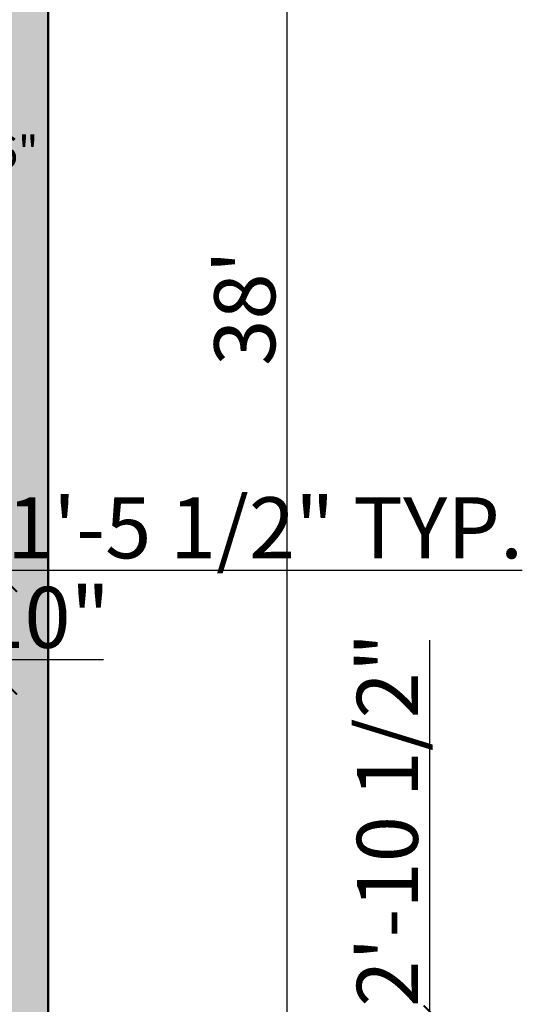
# Model space of a CAD drawing. Units: inches. Extents: x 2419 to 2878, y 1068 to 1713.
# Tile 13 of 20: x 2775 to 2878, y 1207 to 1409. Entities that reach past the tile are written whole.
import ezdxf

# ---------------------------------------------------------------- set-up
doc = ezdxf.new("R2010")
doc.units = ezdxf.units.IN
for name, color, linetype, lineweight in [('A-ANNO-DIMS', 2, 'Continuous', 18), ('A-AREA-IDEN', 7, 'Continuous', 18), ('A-FLOR-PRKG-PATT', 1, 'Continuous', 13), ('A-FURN-PATT', 254, 'Continuous', 13), ('A-WALL', 7, 'Continuous', 50)]:
    doc.layers.add(name, color=color, linetype=linetype, lineweight=lineweight)
doc.layers.add('A-FLOR-FIXT-PATT', color=254, linetype='Continuous', lineweight=13, true_color=0xd7ebd2)
doc.layers.add('A-WALL-PATT', color=18, linetype='Continuous', lineweight=13, true_color=0x000000)
doc.styles.get("Standard").update_dxf_attribs({"font": 'arial.ttf'})
doc.dimstyles.new('ISO-25', dxfattribs={"dimtxt": 12.5, "dimasz": 2.5, "dimexe": 1.25, "dimexo": 0.625, "dimtad": 1, "dimdec": 0, "dimlunit": 4, "dimtxsty": 'Standard', "dimblk": 'ARCHTICK', "dimcen": 2.5, "dimse1": 1, "dimse2": 1, "dimclrd": 4, "dimadec": 0, "dimazin": 0, "dimtfac": 1, "dimtdec": 0, "dimtmove": 0, "dimatfit": 3, "dimfxl": 1, "dimarcsym": 0})

# ---------------------------------------------------------------- blocks, each defined once
blk = doc.blocks.new('_ArchTick')
at = {"color": 0, "linetype": 'ByBlock', "const_width": 0.15}
blk.add_lwpolyline([(-0.5, -0.5), (0.5, 0.5)], dxfattribs=at)
blk = doc.blocks.new('*D17')
at = {"layer": 'A-ANNO-DIMS', "color": 0, "lineweight": -2, "transparency": 16777216}
blk.add_line((2829.44, 1577.81), (2829.44, 1121.81), dxfattribs=at)
at = {"layer": 'Defpoints', "color": 0, "transparency": 16777216}
for p in [(2780.51, 1577.81), (2780.51, 1121.81), (2829.44, 1121.81)]:
    blk.add_point(p, dxfattribs=at)
at = {"layer": 'A-ANNO-DIMS', "color": 0, "lineweight": -2, "transparency": 16777216, "xscale": 2.5, "yscale": 2.5, "zscale": 2.5}
for p, rotation in [((2829.44, 1577.81), 90), ((2829.44, 1121.81), 270)]:
    blk.add_blockref('_ArchTick', p, dxfattribs=dict(at, rotation=rotation))
at = {"layer": 'A-ANNO-DIMS', "color": 0, "transparency": 16777216, "insert": (2822.42, 1349.81), "char_height": 12.5, "attachment_point": 5, "rotation": 90}
blk.add_mtext("38'", dxfattribs=at)
blk = doc.blocks.new('*D18')
at = {"layer": 'A-ANNO-DIMS', "color": 4, "lineweight": -2, "transparency": 16777216}
for p, q in [((2772.91, 1292.99), (2772.91, 1271.99)), ((2772.91, 1271.99), (2772.91, 1133))]:
    blk.add_line(p, q, dxfattribs=at)
at = {"layer": 'Defpoints', "color": 0, "transparency": 16777216}
for p in [(2769.76, 1292.99), (2769.76, 1271.99), (2772.91, 1271.99)]:
    blk.add_point(p, dxfattribs=at)
at = {"layer": 'A-ANNO-DIMS', "color": 4, "lineweight": -2, "transparency": 16777216, "xscale": 2.5, "yscale": 2.5, "zscale": 2.5}
for p, rotation in [((2772.91, 1292.99), 90), ((2772.91, 1271.99), 270)]:
    blk.add_blockref('_ArchTick', p, dxfattribs=dict(at, rotation=rotation))
at = {"layer": 'A-ANNO-DIMS', "color": 0, "transparency": 16777216, "insert": (2765.82, 1201.24), "char_height": 12.5, "attachment_point": 5, "rotation": 90}
blk.add_mtext('CHAIR 1\'-9" TYP.', dxfattribs=at)
blk = doc.blocks.new('*D19')
at = {"layer": 'A-ANNO-DIMS', "color": 4, "lineweight": -2, "transparency": 16777216}
for p, q in [((2752.42, 1296.14), (2769.76, 1296.14)), ((2769.76, 1296.14), (2877.65, 1296.14))]:
    blk.add_line(p, q, dxfattribs=at)
at = {"layer": 'Defpoints', "color": 0, "transparency": 16777216}
for p in [(2769.76, 1296.14), (2752.42, 1292.99), (2769.76, 1292.99)]:
    blk.add_point(p, dxfattribs=at)
at = {"layer": 'A-ANNO-DIMS', "color": 4, "lineweight": -2, "transparency": 16777216, "xscale": 2.5, "yscale": 2.5, "zscale": 2.5, "rotation": 180}
blk.add_blockref('_ArchTick', (2752.42, 1296.14), dxfattribs=at)
at = {"layer": 'A-ANNO-DIMS', "color": 4, "lineweight": -2, "transparency": 16777216, "xscale": 2.5, "yscale": 2.5, "zscale": 2.5}
blk.add_blockref('_ArchTick', (2769.76, 1296.14), dxfattribs=at)
at = {"layer": 'A-ANNO-DIMS', "color": 0, "transparency": 16777216, "insert": (2824.95, 1303.22), "char_height": 12.5, "attachment_point": 5}
blk.add_mtext('1\'-5 1/2" TYP.', dxfattribs=at)
blk = doc.blocks.new('*D33')
at = {"layer": 'A-ANNO-DIMS', "color": 4, "lineweight": -2, "transparency": 16777216}
for p, q in [((2710.85, 1277.89), (2744.94, 1277.89)), ((2744.94, 1277.89), (2791.85, 1277.89))]:
    blk.add_line(p, q, dxfattribs=at)
at = {"layer": 'Defpoints', "color": 0, "transparency": 16777216}
for p in [(2744.94, 1277.89), (2710.85, 1272.77), (2744.94, 1272.77)]:
    blk.add_point(p, dxfattribs=at)
at = {"layer": 'A-ANNO-DIMS', "color": 4, "lineweight": -2, "transparency": 16777216, "xscale": 2.5, "yscale": 2.5, "zscale": 2.5, "rotation": 180}
blk.add_blockref('_ArchTick', (2710.85, 1277.89), dxfattribs=at)
at = {"layer": 'A-ANNO-DIMS', "color": 4, "lineweight": -2, "transparency": 16777216, "xscale": 2.5, "yscale": 2.5, "zscale": 2.5}
blk.add_blockref('_ArchTick', (2744.94, 1277.89), dxfattribs=at)
at = {"layer": 'A-ANNO-DIMS', "color": 0, "transparency": 16777216, "insert": (2769.65, 1284.89), "char_height": 12.5, "attachment_point": 5}
blk.add_mtext('2\'-10"', dxfattribs=at)
blk = doc.blocks.new('*D37')
at = {"layer": 'A-ANNO-DIMS', "color": 4, "lineweight": -2, "transparency": 16777216}
for p, q in [((2736.32, 1605.01), (2771.51, 1605.01)), ((2771.51, 1605.01), (2818.42, 1605.01))]:
    blk.add_line(p, q, dxfattribs=at)
at = {"layer": 'Defpoints', "color": 0, "transparency": 16777216}
for p in [(2771.51, 1605.01), (2736.32, 1205.81), (2771.51, 1205.81)]:
    blk.add_point(p, dxfattribs=at)
at = {"layer": 'A-ANNO-DIMS', "color": 4, "lineweight": -2, "transparency": 16777216, "xscale": 2.5, "yscale": 2.5, "zscale": 2.5, "rotation": 180}
blk.add_blockref('_ArchTick', (2736.32, 1605.01), dxfattribs=at)
at = {"layer": 'A-ANNO-DIMS', "color": 4, "lineweight": -2, "transparency": 16777216, "xscale": 2.5, "yscale": 2.5, "zscale": 2.5}
blk.add_blockref('_ArchTick', (2771.51, 1605.01), dxfattribs=at)
at = {"layer": 'A-ANNO-DIMS', "color": 0, "transparency": 16777216, "insert": (2796.22, 1611.91), "char_height": 12.5, "attachment_point": 5}
blk.add_mtext('2\'-11"', dxfattribs=at)
blk = doc.blocks.new('*D40')
at = {"layer": 'A-ANNO-DIMS', "color": 4, "lineweight": -2, "transparency": 16777216}
for p, q in [((2858.71, 1205.81), (2858.71, 1281.84)), ((2858.71, 1171.28), (2858.71, 1205.81))]:
    blk.add_line(p, q, dxfattribs=at)
at = {"layer": 'Defpoints', "color": 0, "transparency": 16777216}
for p in [(2736.32, 1205.81), (2858.71, 1205.81), (2736.32, 1171.28)]:
    blk.add_point(p, dxfattribs=at)
at = {"layer": 'A-ANNO-DIMS', "color": 4, "lineweight": -2, "transparency": 16777216, "xscale": 2.5, "yscale": 2.5, "zscale": 2.5}
for p, rotation in [((2858.71, 1205.81), 90), ((2858.71, 1171.28), 270)]:
    blk.add_blockref('_ArchTick', p, dxfattribs=dict(at, rotation=rotation))
at = {"layer": 'A-ANNO-DIMS', "color": 0, "transparency": 16777216, "insert": (2851.63, 1245.08), "char_height": 12.5, "attachment_point": 5, "rotation": 90}
blk.add_mtext('2\'-10 1/2"', dxfattribs=at)
blk = doc.blocks.new('*D51')
at = {"layer": 'A-ANNO-DIMS', "color": 4, "lineweight": -2, "transparency": 16777216}
for p, q in [((2738.51, 1079.92), (2771.51, 1079.92)), ((2771.51, 1079.92), (2808.71, 1079.92))]:
    blk.add_line(p, q, dxfattribs=at)
at = {"layer": 'Defpoints', "color": 0, "transparency": 16777216}
for p in [(2738.51, 1447.89), (2771.51, 1437.39), (2771.51, 1079.92)]:
    blk.add_point(p, dxfattribs=at)
at = {"layer": 'A-ANNO-DIMS', "color": 4, "lineweight": -2, "transparency": 16777216, "xscale": 2.5, "yscale": 2.5, "zscale": 2.5, "rotation": 180}
blk.add_blockref('_ArchTick', (2738.51, 1079.92), dxfattribs=at)
at = {"layer": 'A-ANNO-DIMS', "color": 4, "lineweight": -2, "transparency": 16777216, "xscale": 2.5, "yscale": 2.5, "zscale": 2.5}
blk.add_blockref('_ArchTick', (2771.51, 1079.92), dxfattribs=at)
at = {"layer": 'A-ANNO-DIMS', "color": 0, "transparency": 16777216, "insert": (2791.36, 1086.93), "char_height": 12.5, "attachment_point": 5}
blk.add_mtext('2\'-9"', dxfattribs=at)

msp = doc.modelspace()

# ---------------------------------------------------------------- hatches: boundary and pattern name
at = {"layer": 'A-FLOR-FIXT-PATT'}
h = msp.add_hatch(color=256, dxfattribs=at)
h.dxf.hatch_style = 1
h.paths.add_polyline_path([(2771.51, 1458.39), (2763.51, 1458.39), (2763.51, 1437.39), (2771.51, 1437.39)])
h.paths.add_polyline_path([(2770.51, 1456.39, 0.5), (2769.51, 1457.39), (2765.51, 1457.39, 0.5), (2764.51, 1456.39), (2764.51, 1439.39, 0.5), (2765.51, 1438.39), (2769.51, 1438.39, 0.5), (2770.51, 1439.39)], flags=16)
h.paths.add_polyline_path([(2706.38, 1408.81), (2685.38, 1408.81), (2685.38, 1400.81), (2706.38, 1400.81)])
h.paths.add_polyline_path([(2704.38, 1401.81, 0.5), (2705.38, 1402.81), (2705.38, 1406.81, 0.5), (2704.38, 1407.81), (2687.38, 1407.81, 0.5), (2686.38, 1406.81), (2686.38, 1402.81, 0.5), (2687.38, 1401.81)], flags=16)
h.paths.add_polyline_path([(2574.48, 1207.45), (2633.94, 1207.45), (2633.94, 1217.37), (2574.48, 1217.37)], flags=9)
h.paths.add_polyline_path([(2574.45, 1217.83), (2610.47, 1217.83), (2610.47, 1227.88), (2574.45, 1227.88)], flags=9)
h.paths.add_polyline_path([(2672.43, 1304.02), (2718.62, 1304.02), (2718.62, 1313.94), (2672.43, 1313.94)], flags=9)
h.paths.add_polyline_path([(2672.4, 1314.4), (2750.13, 1314.4), (2750.13, 1324.45), (2672.4, 1324.45)], flags=9)
h.paths.add_polyline_path([(2500.43, 1374.44), (2544.8, 1374.44), (2544.8, 1384.36), (2500.43, 1384.36)], flags=9)
h.paths.add_polyline_path([(2500.41, 1384.82), (2566.08, 1384.82), (2566.08, 1394.87), (2500.41, 1394.87)], flags=9)
h.paths.add_polyline_path([(2738.93, 1376.75), (2778.27, 1376.75), (2778.27, 1386.67), (2738.93, 1386.67)], flags=9)
h.paths.add_polyline_path([(2659.12, 1357.8), (2703.49, 1357.8), (2703.49, 1367.72), (2659.12, 1367.72)], flags=9)
h.paths.add_polyline_path([(2659.1, 1368.18), (2694.11, 1368.18), (2694.11, 1378.23), (2659.1, 1378.23)], flags=9)
h.paths.add_polyline_path([(2730.12, 1466.07), (2769.46, 1466.07), (2769.46, 1475.99), (2730.12, 1475.99)], flags=9)
h.paths.add_polyline_path([(2730.1, 1476.45), (2765.12, 1476.45), (2765.12, 1486.5), (2730.1, 1486.5)], flags=9)
h.paths.add_polyline_path([(2730.38, 1518.65), (2761.48, 1518.65), (2761.48, 1528.57), (2730.38, 1528.57)], flags=9)
h.paths.add_polyline_path([(2730.36, 1529.03), (2780.96, 1529.03), (2780.96, 1539.07), (2730.36, 1539.07)], flags=9)
h.paths.add_polyline_path([(2629.32, 1455.19), (2688.78, 1455.19), (2688.78, 1465.11), (2629.32, 1465.11)], flags=9)
h.paths.add_polyline_path([(2629.3, 1465.57), (2681.9, 1465.57), (2681.9, 1475.62), (2629.3, 1475.62)], flags=9)
h.paths.add_polyline_path([(2513.23, 1456.48), (2562.63, 1456.48), (2562.63, 1466.4), (2513.23, 1466.4)], flags=9)
h.paths.add_polyline_path([(2513.21, 1466.86), (2556.26, 1466.86), (2556.26, 1476.91), (2513.21, 1476.91)], flags=9)
h.paths.add_polyline_path([(2488.87, 1521.54), (2519.97, 1521.54), (2519.97, 1531.46), (2488.87, 1531.46)], flags=9)
h.paths.add_polyline_path([(2536.55, 1543.51), (2580.92, 1543.51), (2580.92, 1553.43), (2536.55, 1553.43)], flags=9)
h.paths.add_polyline_path([(2536.56, 1553.92), (2573.53, 1553.92), (2573.53, 1563.8), (2536.56, 1563.8)], flags=9)
at = {"layer": 'A-FLOR-PRKG-PATT'}
h = msp.add_hatch(color=256, dxfattribs=at)
h.dxf.hatch_style = 1
edge = h.paths.add_edge_path()
edge.add_ellipse((2561.37, 1279.45), major_axis=(3.99, 0), ratio=0.842304, start_angle=0.6466, end_angle=90)
edge.add_line((2561.37, 1282.81), (2511.57, 1282.81))
edge.add_ellipse((2511.57, 1279.45), major_axis=(3.99, 0), ratio=0.842304, start_angle=90, end_angle=179.3534)
edge.add_ellipse((10560.89, 1188.62), major_axis=(-8054.03, 0), ratio=0.8423039, start_angle=-0.646554, end_angle=-0.628237)
edge.add_ellipse((2509.23, 1276.91), major_axis=(1.69, 0), ratio=0.842304, start_angle=179.3718, end_angle=248.4648)
edge.add_ellipse((10560.33, 1188.62), major_axis=(8052.29, 0), ratio=0.8423039, start_angle=179.353446, end_angle=179.381357, ccw=False)
edge.add_ellipse((2511.01, 1279.45), major_axis=(2.25, 0), ratio=0.842304, start_angle=90, end_angle=179.3534, ccw=False)
edge.add_line((2511.01, 1281.35), (2561.94, 1281.35))
edge.add_ellipse((2561.94, 1279.45), major_axis=(-2.25, 0), ratio=0.842304, start_angle=180.6466, end_angle=270, ccw=False)
edge.add_ellipse((-5487.38, 1188.62), major_axis=(8052.29, 0), ratio=0.8423039, start_angle=0.528271, end_angle=0.646554, ccw=False)
edge.add_ellipse((2563.71, 1276.91), major_axis=(-1.69, 0), ratio=0.842304, start_angle=111.5352, end_angle=180.6282)
edge.add_ellipse((-5487.95, 1188.62), major_axis=(-8054.03, 0), ratio=0.8423039, start_angle=180.628237, end_angle=180.646554)
edge = h.paths.add_edge_path()
edge.add_ellipse((2564.91, 1261.91), major_axis=(-1.12, 0), ratio=0.842304, start_angle=180, end_angle=270)
edge.add_line((2564.91, 1262.86), (2564.43, 1262.86))
edge.add_ellipse((-5487.38, 1188.62), major_axis=(8052.29, 0), ratio=0.8423039, start_angle=0.383867, end_angle=0.528271, ccw=False)
edge.add_line((2564.65, 1242.56), (2564.91, 1242.56))
edge.add_ellipse((2564.91, 1243.51), major_axis=(-1.12, 0), ratio=0.842304, start_angle=90, end_angle=180)
edge.add_line((2566.03, 1243.51), (2566.03, 1261.91))
edge = h.paths.add_edge_path()
edge.add_ellipse((2564.91, 1174.99), major_axis=(1.12, 0), ratio=0.842304, start_angle=0, end_angle=90)
edge.add_line((2564.91, 1175.94), (2564.89, 1175.94))
edge.add_ellipse((-5487.38, 1188.62), major_axis=(8052.29, 0), ratio=0.8423039, start_angle=-0.134987, end_angle=-0.090229, ccw=False)
edge.add_ellipse((2163.34, 1170.91), major_axis=(401.54, 0), ratio=0.842304, start_angle=-2.18, end_angle=-0.1356, ccw=False)
edge.add_line((2564.47, 1155.64), (2564.91, 1155.64))
edge.add_ellipse((2564.91, 1156.59), major_axis=(-1.12, 0), ratio=0.842304, start_angle=90, end_angle=180)
edge.add_line((2566.03, 1156.59), (2566.03, 1174.99))
h.paths.add_polyline_path([(2574.48, 1207.45), (2633.94, 1207.45), (2633.94, 1217.37), (2574.48, 1217.37)], flags=9)
h.paths.add_polyline_path([(2574.45, 1217.83), (2610.47, 1217.83), (2610.47, 1227.88), (2574.45, 1227.88)], flags=9)
h.paths.add_polyline_path([(2672.43, 1304.02), (2718.62, 1304.02), (2718.62, 1313.94), (2672.43, 1313.94)], flags=9)
h.paths.add_polyline_path([(2672.4, 1314.4), (2750.13, 1314.4), (2750.13, 1324.45), (2672.4, 1324.45)], flags=9)
h.paths.add_polyline_path([(2500.43, 1374.44), (2544.8, 1374.44), (2544.8, 1384.36), (2500.43, 1384.36)], flags=9)
h.paths.add_polyline_path([(2500.41, 1384.82), (2566.08, 1384.82), (2566.08, 1394.87), (2500.41, 1394.87)], flags=9)
h.paths.add_polyline_path([(2738.93, 1376.75), (2778.27, 1376.75), (2778.27, 1386.67), (2738.93, 1386.67)], flags=9)
h.paths.add_polyline_path([(2659.12, 1357.8), (2703.49, 1357.8), (2703.49, 1367.72), (2659.12, 1367.72)], flags=9)
h.paths.add_polyline_path([(2659.1, 1368.18), (2694.11, 1368.18), (2694.11, 1378.23), (2659.1, 1378.23)], flags=9)
h.paths.add_polyline_path([(2730.12, 1466.07), (2769.46, 1466.07), (2769.46, 1475.99), (2730.12, 1475.99)], flags=9)
h.paths.add_polyline_path([(2730.1, 1476.45), (2765.12, 1476.45), (2765.12, 1486.5), (2730.1, 1486.5)], flags=9)
h.paths.add_polyline_path([(2730.38, 1518.65), (2761.48, 1518.65), (2761.48, 1528.57), (2730.38, 1528.57)], flags=9)
h.paths.add_polyline_path([(2730.36, 1529.03), (2780.96, 1529.03), (2780.96, 1539.07), (2730.36, 1539.07)], flags=9)
h.paths.add_polyline_path([(2629.32, 1455.19), (2688.78, 1455.19), (2688.78, 1465.11), (2629.32, 1465.11)], flags=9)
h.paths.add_polyline_path([(2629.3, 1465.57), (2681.9, 1465.57), (2681.9, 1475.62), (2629.3, 1475.62)], flags=9)
h.paths.add_polyline_path([(2513.23, 1456.48), (2562.63, 1456.48), (2562.63, 1466.4), (2513.23, 1466.4)], flags=9)
h.paths.add_polyline_path([(2513.21, 1466.86), (2556.26, 1466.86), (2556.26, 1476.91), (2513.21, 1476.91)], flags=9)
h.paths.add_polyline_path([(2488.87, 1521.54), (2519.97, 1521.54), (2519.97, 1531.46), (2488.87, 1531.46)], flags=9)
h.paths.add_polyline_path([(2536.55, 1543.51), (2580.92, 1543.51), (2580.92, 1553.43), (2536.55, 1553.43)], flags=9)
h.paths.add_polyline_path([(2536.56, 1553.92), (2573.53, 1553.92), (2573.53, 1563.8), (2536.56, 1563.8)], flags=9)
at = {"layer": 'A-FURN-PATT'}
h = msp.add_hatch(color=256, dxfattribs=at)
h.dxf.hatch_style = 1
h.paths.add_polyline_path([(2710.17, 1562.64), (2707.17, 1559.64), (2709.17, 1559.64, -0.414214), (2710.17, 1560.64)])
h.paths.add_polyline_path([(2711.17, 1559.64, 1), (2709.17, 1559.64, 1)])
h.paths.add_polyline_path([(2710.17, 1562.64), (2710.17, 1560.64, -0.414214), (2711.17, 1559.64), (2713.17, 1559.64)])
h.paths.add_polyline_path([(2713.17, 1559.64), (2711.17, 1559.64, -0.414214), (2710.17, 1558.64), (2710.17, 1556.64)])
h.paths.add_polyline_path([(2710.17, 1558.64, -0.414214), (2709.17, 1559.64), (2707.17, 1559.64), (2710.17, 1556.64)])
h.paths.add_polyline_path([(2613.13, 1558.89, 1), (2611.13, 1558.89, 1)])
h.paths.add_polyline_path([(2612.13, 1561.89), (2612.13, 1559.89, -0.414214), (2613.13, 1558.89), (2615.13, 1558.89)])
h.paths.add_polyline_path([(2612.13, 1559.89), (2612.13, 1561.89), (2609.13, 1558.89), (2611.13, 1558.89, -0.414214)])
h.paths.add_polyline_path([(2612.13, 1557.89, -0.414214), (2611.13, 1558.89), (2609.13, 1558.89), (2612.13, 1555.89)])
h.paths.add_polyline_path([(2574.48, 1207.45), (2633.94, 1207.45), (2633.94, 1217.37), (2574.48, 1217.37)], flags=9)
h.paths.add_polyline_path([(2574.45, 1217.83), (2610.47, 1217.83), (2610.47, 1227.88), (2574.45, 1227.88)], flags=9)
h.paths.add_polyline_path([(2672.43, 1304.02), (2718.62, 1304.02), (2718.62, 1313.94), (2672.43, 1313.94)], flags=9)
h.paths.add_polyline_path([(2672.4, 1314.4), (2750.13, 1314.4), (2750.13, 1324.45), (2672.4, 1324.45)], flags=9)
h.paths.add_polyline_path([(2500.43, 1374.44), (2544.8, 1374.44), (2544.8, 1384.36), (2500.43, 1384.36)], flags=9)
h.paths.add_polyline_path([(2500.41, 1384.82), (2566.08, 1384.82), (2566.08, 1394.87), (2500.41, 1394.87)], flags=9)
h.paths.add_polyline_path([(2738.93, 1376.75), (2778.27, 1376.75), (2778.27, 1386.67), (2738.93, 1386.67)], flags=9)
h.paths.add_polyline_path([(2659.12, 1357.8), (2703.49, 1357.8), (2703.49, 1367.72), (2659.12, 1367.72)], flags=9)
h.paths.add_polyline_path([(2659.1, 1368.18), (2694.11, 1368.18), (2694.11, 1378.23), (2659.1, 1378.23)], flags=9)
h.paths.add_polyline_path([(2730.12, 1466.07), (2769.46, 1466.07), (2769.46, 1475.99), (2730.12, 1475.99)], flags=9)
h.paths.add_polyline_path([(2730.1, 1476.45), (2765.12, 1476.45), (2765.12, 1486.5), (2730.1, 1486.5)], flags=9)
h.paths.add_polyline_path([(2730.38, 1518.65), (2761.48, 1518.65), (2761.48, 1528.57), (2730.38, 1528.57)], flags=9)
h.paths.add_polyline_path([(2730.36, 1529.03), (2780.96, 1529.03), (2780.96, 1539.07), (2730.36, 1539.07)], flags=9)
h.paths.add_polyline_path([(2629.32, 1455.19), (2688.78, 1455.19), (2688.78, 1465.11), (2629.32, 1465.11)], flags=9)
h.paths.add_polyline_path([(2629.3, 1465.57), (2681.9, 1465.57), (2681.9, 1475.62), (2629.3, 1475.62)], flags=9)
h.paths.add_polyline_path([(2513.23, 1456.48), (2562.63, 1456.48), (2562.63, 1466.4), (2513.23, 1466.4)], flags=9)
h.paths.add_polyline_path([(2513.21, 1466.86), (2556.26, 1466.86), (2556.26, 1476.91), (2513.21, 1476.91)], flags=9)
h.paths.add_polyline_path([(2488.87, 1521.54), (2519.97, 1521.54), (2519.97, 1531.46), (2488.87, 1531.46)], flags=9)
h.paths.add_polyline_path([(2536.55, 1543.51), (2580.92, 1543.51), (2580.92, 1553.43), (2536.55, 1553.43)], flags=9)
h.paths.add_polyline_path([(2536.56, 1553.92), (2573.53, 1553.92), (2573.53, 1563.8), (2536.56, 1563.8)], flags=9)
at = {"layer": 'A-WALL-PATT'}
h = msp.add_hatch(color=256, dxfattribs=at)
h.dxf.hatch_style = 1
h.paths.add_polyline_path([(2780.51, 1577.81), (2471.51, 1577.81), (2471.51, 1121.81), (2780.51, 1121.81)])
h.paths.add_polyline_path([(2480.51, 1568.81), (2771.51, 1568.81), (2771.51, 1130.81), (2480.51, 1130.81)], flags=16)
h.paths.add_polyline_path([(2528.51, 1568.81), (2528.51, 1512.81), (2594.51, 1512.81), (2594.51, 1414.81), (2596.57, 1414.81), (2596.57, 1441.61), (2597.82, 1441.61), (2597.82, 1441.58, -0.384016), (2625.03, 1414.81), (2725.51, 1414.81), (2725.51, 1567.55), (2728.3, 1567.55), (2746.89, 1567.55), (2746.89, 1566.73), (2746.87, 1566.73, -0.367216), (2730.51, 1549.09), (2730.51, 1512.81), (2750.85, 1512.81), (2750.85, 1510.03, -0.401453), (2733.08, 1491.46), (2733.08, 1491.44), (2732.27, 1491.44), (2732.27, 1507.81), (2730.51, 1507.81), (2730.51, 1408.81), (2736.51, 1408.81), (2736.51, 1349.81), (2632.51, 1349.81), (2632.51, 1408.81), (2528.51, 1408.81), (2528.51, 1414.81), (2503.97, 1414.81), (2503.97, 1494.85), (2558.38, 1494.85), (2558.38, 1507.81), (2529.96, 1507.81, -0.414214), (2530.82, 1506.96), (2530.82, 1497.26, -0.414214), (2529.96, 1496.4), (2514.56, 1496.4, -0.414214), (2513.7, 1497.26), (2513.7, 1506.96, -0.414214), (2514.56, 1507.81), (2528.51, 1507.81), (2528.51, 1512.81), (2480.51, 1512.81)], flags=0)
h.paths.add_polyline_path([(2516.26, 1507.81), (2528.26, 1507.81), (2528.26, 1505.81), (2523.42, 1505.81), (2524.07, 1504.67), (2529.39, 1504.67, -0.414214), (2529.96, 1504.1), (2529.96, 1497.83, -0.414214), (2529.39, 1497.26), (2515.13, 1497.26, -0.414214), (2514.56, 1497.83), (2514.56, 1504.1, -0.414214), (2515.13, 1504.67), (2520.69, 1504.67), (2521.34, 1505.81), (2516.26, 1505.81)], flags=0)
h.paths.add_polyline_path([(2522.02, 1505.53), (2522.82, 1507.32, -0.65506), (2522.25, 1506.06), (2522.19, 1505.93), (2522.43, 1505.53)], flags=0)
h.paths.add_polyline_path([(2522.83, 1500.97, -1), (2521.69, 1500.97, -1)], flags=0)
h.paths.add_polyline_path([(2522.55, 1500.97, -1), (2521.98, 1500.97, -1)], flags=0)
h.paths.add_polyline_path([(2482.01, 1470.63), (2499.89, 1470.63), (2499.89, 1448.27), (2482.01, 1448.27), (2482.01, 1452.74), (2481.26, 1452.74), (2481.26, 1449.76), (2480.51, 1449.76), (2480.51, 1469.14), (2481.26, 1469.14), (2481.26, 1466.16), (2482.01, 1466.16)], flags=0)
h.paths.add_polyline_path([(2488.71, 1466.16, -1), (2484.24, 1466.16, -1)], flags=0)
h.paths.add_polyline_path([(2496.17, 1466.16, -1), (2490.2, 1466.16, -1)], flags=0)
h.paths.add_polyline_path([(2487.97, 1466.16, -1), (2484.99, 1466.16, -1)], flags=0)
h.paths.add_polyline_path([(2495.42, 1466.16, -1), (2490.95, 1466.16, -1)], flags=0)
h.paths.add_polyline_path([(2487.22, 1466.16, -1), (2485.73, 1466.16, -1)], flags=0)
h.paths.add_polyline_path([(2494.68, 1466.16, -1), (2491.69, 1466.16, -1)], flags=0)
h.paths.add_polyline_path([(2499.11, 1468, -1), (2497.98, 1468, -1)], flags=0)
h.paths.add_polyline_path([(2493.93, 1466.16, -1), (2492.44, 1466.16, -1)], flags=0)
h.paths.add_polyline_path([(2499.37, 1463.71, -1), (2498.17, 1463.71, -1)], flags=0)
h.paths.add_polyline_path([(2484.24, 1461.69), (2496.17, 1461.69), (2496.17, 1457.22), (2484.24, 1457.22)], flags=0)
h.paths.add_polyline_path([(2484.99, 1460.94), (2495.42, 1460.94), (2495.42, 1457.96), (2484.99, 1457.96)], flags=0)
h.paths.add_polyline_path([(2586.88, 1510.03), (2587.69, 1510.03), (2587.69, 1491.44), (2586.88, 1491.44)], flags=0)
h.paths.add_polyline_path([(2499.26, 1459.41, -1), (2498.2, 1459.41, -1)], flags=0)
h.paths.add_polyline_path([(2489.46, 1452.74, -1), (2483.5, 1452.74, -1)], flags=0)
h.paths.add_polyline_path([(2557.3, 1408.81), (2557.3, 1413.09, -0.401453), (2584.57, 1441.58), (2584.57, 1441.61), (2585.82, 1441.61), (2585.82, 1413.09), (2585.82, 1408.81)], flags=0)
h.paths.add_polyline_path([(2488.71, 1452.74, -1), (2484.24, 1452.74, -1)], flags=0)
h.paths.add_polyline_path([(2495.42, 1452.74, -1), (2490.95, 1452.74, -1)], flags=0)
h.paths.add_polyline_path([(2487.97, 1452.74, -1), (2484.99, 1452.74, -1)], flags=0)
h.paths.add_polyline_path([(2494.68, 1452.74, -1), (2491.69, 1452.74, -1)], flags=0)
h.paths.add_polyline_path([(2487.22, 1452.74, -1), (2485.73, 1452.74, -1)], flags=0)
h.paths.add_polyline_path([(2499.18, 1454.44, -1), (2497.9, 1454.44, -1)], flags=0)
h.paths.add_polyline_path([(2493.93, 1452.74, -1), (2492.44, 1452.74, -1)], flags=0)
h.paths.add_polyline_path([(2499.3, 1450.64, -1), (2497.79, 1450.64, -1)], flags=0)
h.paths.add_polyline_path([(2619.13, 1558.89, -1), (2605.13, 1558.89, -1)], flags=0)
h.paths.add_polyline_path([(2609.13, 1558.89), (2612.13, 1561.89), (2615.13, 1558.89), (2612.13, 1555.89)], flags=0)
h.paths.add_polyline_path([(2611.13, 1558.89, -1), (2613.13, 1558.89, -1)], flags=0)
h.paths.add_polyline_path([(2633.68, 1568.81), (2693.68, 1568.81), (2693.68, 1488.81), (2633.68, 1488.81)], flags=0)
h.paths.add_polyline_path([(2641.68, 1554.41), (2641.68, 1567.61), (2662.48, 1567.61), (2662.48, 1554.41), (2664.88, 1554.41), (2664.88, 1567.61), (2685.68, 1567.61), (2685.68, 1552.41), (2680.48, 1552.41), (2693.68, 1539.21), (2678.48, 1539.21), (2678.48, 1554.41)], flags=0)
h.paths.add_polyline_path([(2637.51, 1408.81), (2731.51, 1408.81), (2731.51, 1354.81), (2637.51, 1354.81), (2637.51, 1357.98), (2635.3, 1357.98), (2635.3, 1358.79), (2637.51, 1358.79)], flags=0)
h.paths.add_polyline_path([(2717.17, 1559.64, -1), (2703.17, 1559.64, -1)], flags=0)
h.paths.add_polyline_path([(2707.17, 1559.64), (2710.17, 1562.64), (2713.17, 1559.64), (2710.17, 1556.64)], flags=0)
h.paths.add_polyline_path([(2709.17, 1559.64, -1), (2711.17, 1559.64, -1)], flags=0)
h.paths.add_polyline_path([(2685.38, 1408.81), (2706.38, 1408.81), (2706.38, 1400.81), (2699.88, 1400.81), (2701.88, 1394.81, -0.501323), (2696.92, 1375.95, -0.132891), (2694.83, 1375.95, -0.501317), (2689.88, 1394.81), (2691.88, 1400.81), (2688.88, 1400.81), (2688.88, 1399.31), (2685.88, 1399.31), (2685.88, 1400.31), (2687.88, 1400.31), (2687.88, 1400.81), (2685.38, 1400.81)], flags=0)
h.paths.add_polyline_path([(2687.38, 1407.81), (2704.38, 1407.81, -0.5), (2705.38, 1406.81), (2705.38, 1402.81, -0.5), (2704.38, 1401.81), (2687.38, 1401.81, -0.5), (2686.38, 1402.81), (2686.38, 1406.81, -0.5)], flags=0)
h.paths.add_polyline_path([(2639.51, 1205.81), (2634.51, 1205.81), (2634.51, 1293.81), (2637.51, 1293.81), (2639.51, 1293.81)], flags=0)
h.paths.add_polyline_path([(2691.88, 1394.81), (2699.88, 1394.81, -0.48008), (2697.52, 1377.29, -0.215004), (2694.23, 1377.29, -0.48008)], flags=0)
h.paths.add_polyline_path([(2757.51, 1453.89), (2763.51, 1451.89), (2763.51, 1454.89), (2762.01, 1454.89), (2762.01, 1457.89), (2763.01, 1457.89), (2763.01, 1455.89), (2763.51, 1455.89), (2763.51, 1458.39), (2771.51, 1458.39), (2771.51, 1437.39), (2763.51, 1437.39), (2763.51, 1443.89), (2757.51, 1441.89, -0.501323), (2738.65, 1446.85, -0.132891), (2738.65, 1448.94, -0.501317)], flags=0)
h.paths.add_polyline_path([(2739.99, 1449.54, -0.48008), (2757.51, 1451.89), (2757.51, 1443.89, -0.48008), (2739.99, 1446.25, -0.215004)], flags=0)
h.paths.add_polyline_path([(2765.51, 1457.39), (2769.51, 1457.39, -0.5), (2770.51, 1456.39), (2770.51, 1439.39, -0.5), (2769.51, 1438.39), (2765.51, 1438.39, -0.5), (2764.51, 1439.39), (2764.51, 1456.39, -0.5)], flags=0)
h = msp.add_hatch(color=256, dxfattribs=at)
h.dxf.hatch_style = 1
h.paths.add_polyline_path([(2771.51, 1354.81), (2736.51, 1354.81), (2736.51, 1408.81), (2771.51, 1408.81), (2771.51, 1414.81), (2625.03, 1414.81, -0.015108), (2625.09, 1413.09), (2625.09, 1408.81), (2632.51, 1408.81), (2632.51, 1376.56), (2635.3, 1376.56, -0.029838), (2637.51, 1376.43), (2637.51, 1408.81), (2731.51, 1408.81), (2731.51, 1354.81), (2637.51, 1354.81), (2637.51, 1357.98), (2635.3, 1357.98), (2632.51, 1357.98), (2632.51, 1349.81), (2771.51, 1349.81)])
h.paths.add_polyline_path([(2639.51, 1298.81), (2637.51, 1298.81), (2480.51, 1298.81), (2480.51, 1293.81), (2637.51, 1293.81), (2639.51, 1293.81)])
h.paths.add_polyline_path([(2639.51, 1293.81), (2637.51, 1293.81), (2634.51, 1293.81), (2634.51, 1244.65), (2638.79, 1244.65, -0.006332), (2639.51, 1244.64)])
h.paths.add_polyline_path([(2639.51, 1205.81), (2771.51, 1205.81), (2771.51, 1210.81), (2639.51, 1210.81), (2639.51, 1216.13), (2638.79, 1216.13), (2634.51, 1216.13), (2634.51, 1130.81), (2639.51, 1130.81)])
h.paths.add_polyline_path([(2596.57, 1413.09), (2596.57, 1414.81), (2585.82, 1414.81), (2585.82, 1413.09), (2585.82, 1408.81), (2596.57, 1408.81)])
h.paths.add_polyline_path([(2557.3, 1413.09, -0.015108), (2557.35, 1414.81), (2480.51, 1414.81), (2480.51, 1408.81), (2557.3, 1408.81)])
h.paths.add_polyline_path([(2574.48, 1207.45), (2633.94, 1207.45), (2633.94, 1217.37), (2574.48, 1217.37)], flags=9)
h.paths.add_polyline_path([(2574.45, 1217.83), (2610.47, 1217.83), (2610.47, 1227.88), (2574.45, 1227.88)], flags=9)
h.paths.add_polyline_path([(2672.43, 1304.02), (2718.62, 1304.02), (2718.62, 1313.94), (2672.43, 1313.94)], flags=9)
h.paths.add_polyline_path([(2672.4, 1314.4), (2750.13, 1314.4), (2750.13, 1324.45), (2672.4, 1324.45)], flags=9)
h.paths.add_polyline_path([(2500.43, 1374.44), (2544.8, 1374.44), (2544.8, 1384.36), (2500.43, 1384.36)], flags=9)
h.paths.add_polyline_path([(2500.41, 1384.82), (2566.08, 1384.82), (2566.08, 1394.87), (2500.41, 1394.87)], flags=9)
h.paths.add_polyline_path([(2738.93, 1376.75), (2778.27, 1376.75), (2778.27, 1386.67), (2738.93, 1386.67)], flags=9)
h.paths.add_polyline_path([(2659.12, 1357.8), (2703.49, 1357.8), (2703.49, 1367.72), (2659.12, 1367.72)], flags=25)
h.paths.add_polyline_path([(2659.1, 1368.18), (2694.11, 1368.18), (2694.11, 1378.23), (2659.1, 1378.23)], flags=25)
h.paths.add_polyline_path([(2730.12, 1466.07), (2769.46, 1466.07), (2769.46, 1475.99), (2730.12, 1475.99)], flags=9)
h.paths.add_polyline_path([(2730.1, 1476.45), (2765.12, 1476.45), (2765.12, 1486.5), (2730.1, 1486.5)], flags=9)
h.paths.add_polyline_path([(2730.38, 1518.65), (2761.48, 1518.65), (2761.48, 1528.57), (2730.38, 1528.57)], flags=9)
h.paths.add_polyline_path([(2730.36, 1529.03), (2780.96, 1529.03), (2780.96, 1539.07), (2730.36, 1539.07)], flags=9)
h.paths.add_polyline_path([(2629.32, 1455.19), (2688.78, 1455.19), (2688.78, 1465.11), (2629.32, 1465.11)], flags=9)
h.paths.add_polyline_path([(2629.3, 1465.57), (2681.9, 1465.57), (2681.9, 1475.62), (2629.3, 1475.62)], flags=9)
h.paths.add_polyline_path([(2513.23, 1456.48), (2562.63, 1456.48), (2562.63, 1466.4), (2513.23, 1466.4)], flags=9)
h.paths.add_polyline_path([(2513.21, 1466.86), (2556.26, 1466.86), (2556.26, 1476.91), (2513.21, 1476.91)], flags=9)
h.paths.add_polyline_path([(2488.87, 1521.54), (2519.97, 1521.54), (2519.97, 1531.46), (2488.87, 1531.46)], flags=9)
h.paths.add_polyline_path([(2536.55, 1543.51), (2580.92, 1543.51), (2580.92, 1553.43), (2536.55, 1553.43)], flags=9)
h.paths.add_polyline_path([(2536.56, 1553.92), (2573.53, 1553.92), (2573.53, 1563.8), (2536.56, 1563.8)], flags=9)

# ---------------------------------------------------------------- linework, layer by layer
at = {"layer": 'A-WALL'}
msp.add_lwpolyline([(2471.51, 1577.81), (2780.51, 1577.81), (2780.51, 1121.81), (2471.51, 1121.81)], close=True, dxfattribs=at)

# ---------------------------------------------------------------- texts
at = {"layer": 'A-AREA-IDEN'}
msp.add_text('4\'6"X2\'6"', height=6.475, dxfattribs=at).set_placement((2740.59, 1378.51))

# ---------------------------------------------------------------- dimensions: what is measured, and where the dimension line sits
at = {"layer": 'A-ANNO-DIMS'}
for base, p1, p2, picture, middle in [((2771.51, 1605.01), (2736.32, 1205.81), (2771.51, 1205.81), '*D37', (2796.22, 1611.91)), ((2771.51, 1079.92), (2738.51, 1447.89), (2771.51, 1437.39), '*D51', (2791.36, 1086.93)), ((2744.94, 1277.89), (2710.85, 1272.77), (2744.94, 1272.77), '*D33', (2769.65, 1284.89))]:
    dim = msp.add_linear_dim(base=base, p1=p1, p2=p2, dimstyle='ISO-25', override={"dimdec": 1, "dimlfac": 1, "dimrnd": 0, "dimzin": 1, "dimdsep": 46, "dimlunit": 4, "dimfrac": 2}, dxfattribs=at)
    dim.commit()
    dim.dimension.update_dxf_attribs({"geometry": picture, "text_midpoint": middle})
for base, p1, p2, override, picture, middle in [((2829.44, 1121.81), (2780.51, 1577.81), (2780.51, 1121.81), {"dimclrd": 0, "dimclre": 0, "dimclrt": 0}, '*D17', (2822.42, 1349.81)), ((2858.71, 1205.81), (2736.32, 1171.28), (2736.32, 1205.81), {"dimdec": 1, "dimlfac": 1, "dimrnd": 0, "dimzin": 1, "dimdsep": 46, "dimlunit": 4, "dimfrac": 2}, '*D40', (2851.63, 1245.08))]:
    dim = msp.add_linear_dim(base=base, p1=p1, p2=p2, angle=90, dimstyle='ISO-25', override=override, dxfattribs=at)
    dim.commit()
    dim.dimension.update_dxf_attribs({"geometry": picture, "text_midpoint": middle})
dim = msp.add_linear_dim(base=(2769.76, 1296.14), p1=(2752.42, 1292.99), p2=(2769.76, 1292.99), text='<> TYP.', dimstyle='ISO-25', override={"dimdec": 1, "dimlfac": 1, "dimrnd": 0, "dimzin": 1, "dimdsep": 46, "dimlunit": 4, "dimfrac": 2}, dxfattribs=at)
dim.commit()
dim.dimension.update_dxf_attribs({"geometry": '*D19', "text_midpoint": (2824.95, 1303.22)})
dim = msp.add_linear_dim(base=(2772.91, 1271.99), p1=(2769.76, 1292.99), p2=(2769.76, 1271.99), angle=270, text='CHAIR <> TYP.', dimstyle='ISO-25', override={"dimdec": 1, "dimlfac": 1, "dimrnd": 0, "dimzin": 1, "dimdsep": 46, "dimlunit": 4, "dimfrac": 2}, dxfattribs=at)
dim.commit()
dim.dimension.update_dxf_attribs({"geometry": '*D18', "text_midpoint": (2765.82, 1201.24)})

doc.saveas('drawing.dxf')
